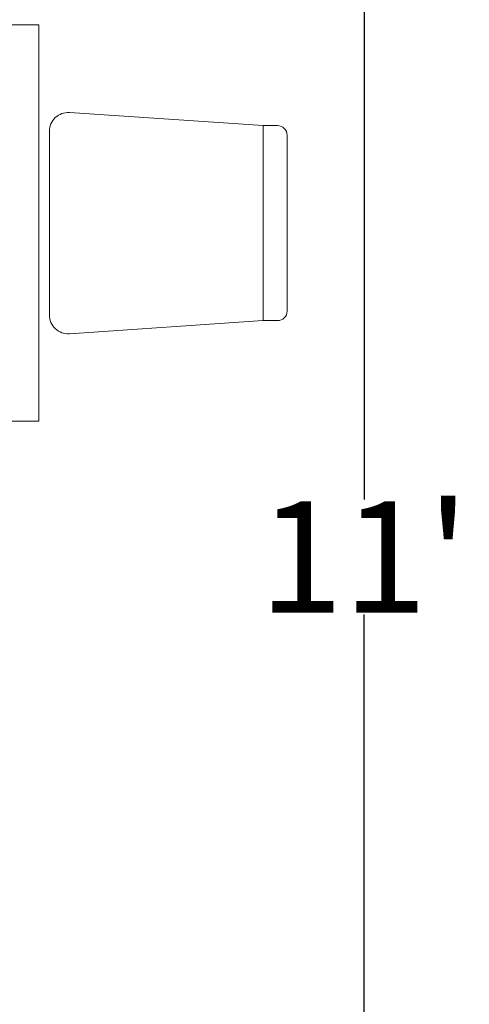
# Model space of a CAD drawing. Units: inches. Extents: x 0 to 281, y -535 to 46.
# Tile 6 of 22: x 198 to 222, y -222 to -168. Entities that reach past the tile are written whole.
import ezdxf

# ---------------------------------------------------------------- set-up
doc = ezdxf.new("R2010")
doc.units = ezdxf.units.IN
doc.header["$MEASUREMENT"] = 0
doc.layers.add('A-ANNO-DIMS', color=2, linetype='Continuous', lineweight=18)
doc.layers.add('A-FURN', color=8, linetype='Continuous', lineweight=18)
doc.styles.get("Standard").update_dxf_attribs({"font": 'arial.ttf'})
doc.dimstyles.get("Standard").update_dxf_attribs({"dimtxt": 0.18, "dimasz": 0.18, "dimexe": 0.18, "dimexo": 0.0625, "dimgap": 0.09, "dimtad": 0, "dimtih": 1, "dimtoh": 1, "dimdec": 0, "dimzin": 0, "dimdsep": 46, "dimlunit": 3, "dimtxsty": 'Standard', "dimcen": 0.09, "dimadec": 0, "dimazin": 0, "dimtfac": 1, "dimtdec": 0, "dimtofl": 0, "dimtmove": 0, "dimatfit": 3, "dimfxl": 1, "dimtolj": 1, "dimtzin": 0, "dimarcsym": 0})

# ---------------------------------------------------------------- blocks, each defined once
blk = doc.blocks.new('*D6')
at = {"layer": 'A-ANNO-DIMS', "color": 0, "lineweight": -2, "transparency": 16777216}
for p, q in [((216.459, -131.591), (216.459, -194.308)), ((216.521, -131.411), (216.639, -131.411)), ((216.459, -263.231), (216.459, -200.513)), ((216.521, -263.411), (216.639, -263.411))]:
    blk.add_line(p, q, dxfattribs=at)
at = {"layer": 'A-ANNO-DIMS', "color": 0, "transparency": 16777216}
for points in [[(216.429, -131.591), (216.489, -131.591), (216.459, -131.411)], [(216.429, -263.231), (216.489, -263.231), (216.459, -263.411)]]:
    blk.add_solid(points, dxfattribs=at)
at = {"layer": 'Defpoints', "color": 0, "transparency": 16777216}
for p in [(216.459, -131.411), (216.459, -263.411), (216.459, -263.411)]:
    blk.add_point(p, dxfattribs=at)
at = {"layer": 'A-ANNO-DIMS', "color": 0, "transparency": 16777216, "insert": (216.459, -197.411), "char_height": 6, "attachment_point": 5}
blk.add_mtext("\\A1;11'", dxfattribs=at)
blk = doc.blocks.new('CHAIR-DINING')
for p, q in [((10.729, 12.842), (1.225, 12.842)), ((0.712, 12.329), (0.712, 11.558)), ((11.243, 11.558), (11.243, 12.329)), ((0, 1.083), (0.712, 11.558)), ((11.243, 11.558), (0.712, 11.558)), ((11.243, 11.558), (11.954, 1.083)), ((1.026, 0), (10.928, 0))]:
    blk.add_line(p, q)
for centre, radius, start, end in [((1.225, 12.329), 0.514, 90, 180), ((10.729, 12.329), 0.514, 0, 90), ((1.026, 1.027), 1.027, 176.8779, 270), ((10.928, 1.027), 1.027, 270, 3.1221)]:
    blk.add_arc(centre, radius, start, end)

msp = doc.modelspace()

# ---------------------------------------------------------------- linework, layer by layer
at = {"layer": 'A-FURN'}
msp.add_lwpolyline([(177.478, -190.086), (177.478, -168.682), (198.882, -168.682), (198.882, -190.086)], close=True, dxfattribs=at)

# ---------------------------------------------------------------- block references
at = {"layer": 'A-FURN', "rotation": 269.9999999981291}
msp.add_blockref('CHAIR-DINING', (199.453, -173.407), dxfattribs=at)

# ---------------------------------------------------------------- dimensions: what is measured, and where the dimension line sits
at = {"layer": 'A-ANNO-DIMS'}
dim = msp.add_linear_dim(base=(216.459, -263.411), p1=(216.459, -131.411), p2=(216.459, -263.411), angle=90, dimstyle='Standard', override={"dimtxt": 6, "dimclrd": 0, "dimclre": 0, "dimclrt": 0}, dxfattribs=at)
dim.commit()
dim.dimension.update_dxf_attribs({"geometry": '*D6', "text_midpoint": (216.459, -197.411)})

doc.saveas('drawing.dxf')
